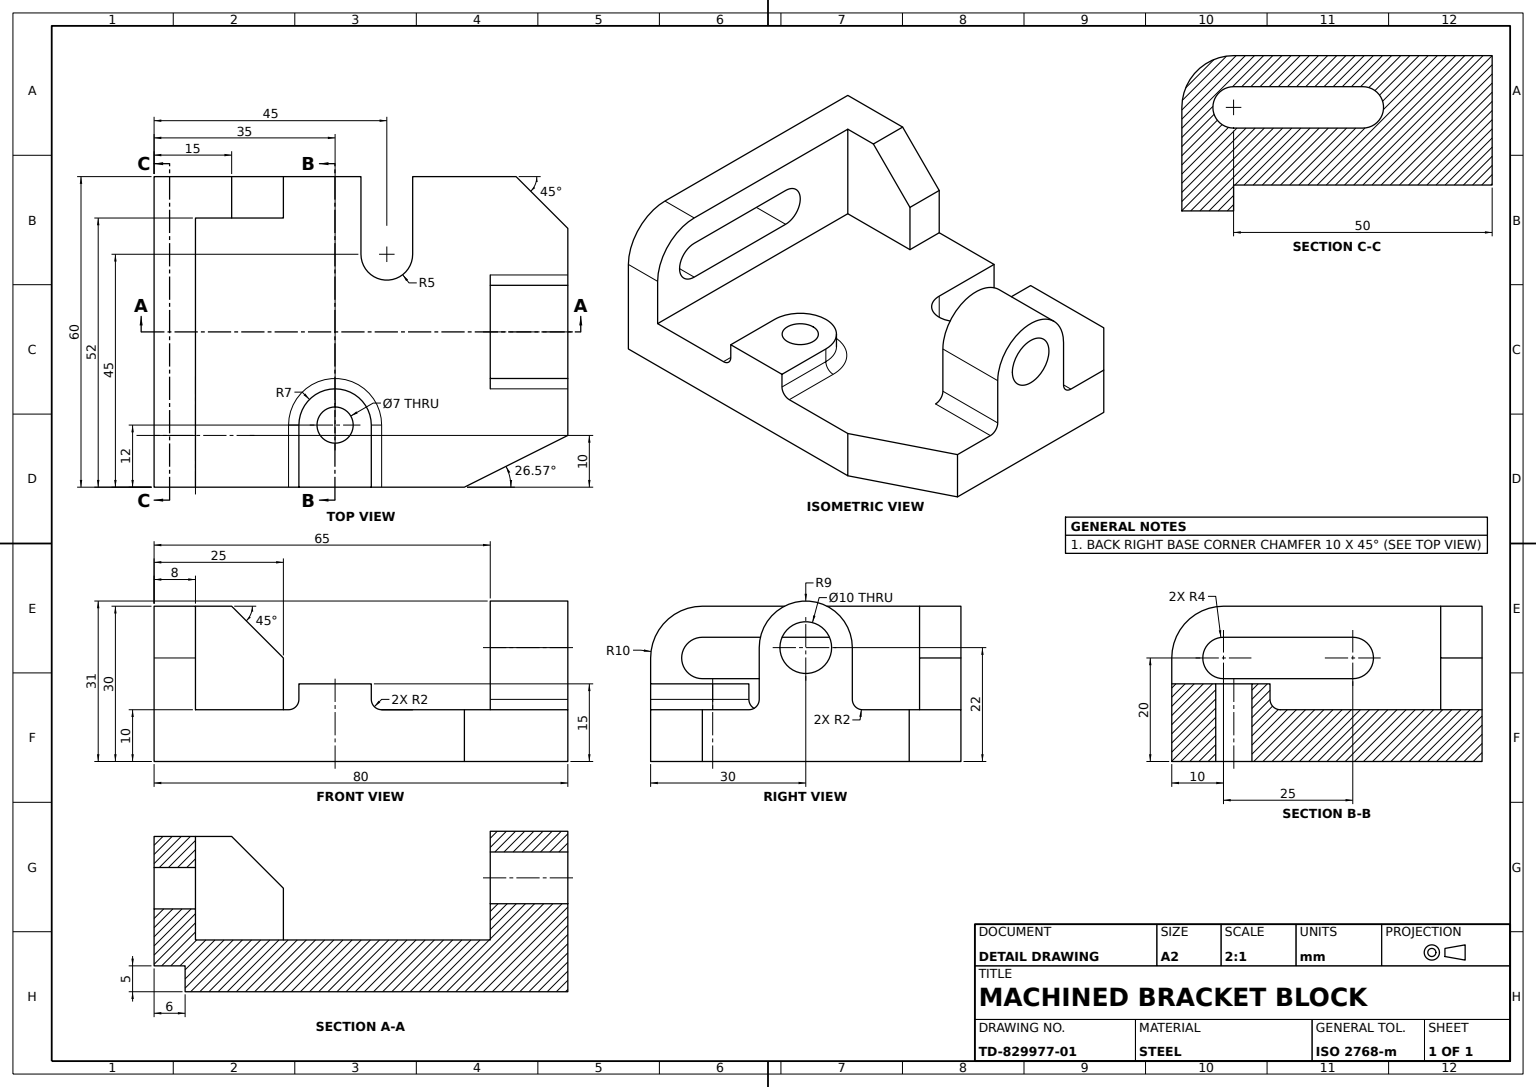
SolidWorks part; units mm, degrees
material "Plain Carbon Steel"
ref_plane "Front Plane" through (0, 0, 0) normal (0, 0, 1) x (1, 0, 0)
ref_plane "Top Plane" through (0, 0, 0) normal (0, 1, 0) x (1, 0, 0)
ref_plane "Right Plane" through (0, 0, 0) normal (1, 0, 0) x (0, 0, -1)
sketch "Base Plate Sketch" plane through (0, 0, 0) normal (0, 1, 0) x (1, 0, 0)
  line L0 (0, 0) -> (0, 30)
  line L1 (0, 30) -> (40, 30)
  line L2 (40, 30) -> (40, 15)
  line L3 (50, 15) -> (50, 30)
  line L4 (50, 30) -> (80, 30)
  line L5 (80, 30) -> (80, -20)
  line L6 (80, -20) -> (60, -30)
  line L7 (60, -30) -> (0, -30)
  line L8 (0, -30) -> (0, 0)
  arc A0 (40, 15) -> (50, 15) centre (45, 15) ccw
  dimension "D3" = 5
  dimension "D1" = 80
  dimension "D2" = 15
  dimension "D4" = 60
  dimension "D5" = 30
  dimension "D6" = 10
  dimension "D7" = 20
  dimension "D8" = 30
extrude "Base Plate 80x60x10" add sketch "Base Plate Sketch" along normal blind 10
chamfer "Base Corner Chamfer 10" distance 10 angle 45 1 edges at (80, 5, -30)
sketch "Slotted Wall Sketch" plane through (0, 0, 0) normal (-1, 0, 0) x (0, 0, 1)
  line L1 (20, 30) -> (-30, 30)
  line L2 (-30, 30) -> (-30, 10)
  line L3 (-30, 10) -> (-30, 0) construction
  line L4 (-30, 10) -> (30, 10)
  line L9 (20, 20) -> (-5, 20) construction
  line L10 (20, 16) -> (-5, 16)
  line L11 (20, 24) -> (-5, 24)
  line L12 (30, 20) -> (30, 10)
  arc A0 (30, 20) -> (20, 30) centre (20, 20) ccw
  arc A1 (20, 16) -> (20, 24) centre (20, 20) ccw
  arc A2 (-5, 24) -> (-5, 16) centre (-5, 20) ccw
  point P18 (7.5, 20)
  dimension "D3" = 10
  dimension "D4" = 4
  dimension "D2" = 20
  dimension "D5" = 10
  dimension "D6" = 25
  dimension "D7" = 12.5
extrude "Slotted Upright Wall" add sketch "Slotted Wall Sketch" against normal blind 8
sketch "Side Block Sketch" plane through (0, 0, -30) normal (0, 0, -1) x (-1, 0, 0)
  line L0 (-8, 30) -> (-25, 30)
  line L1 (-25, 30) -> (-25, 10)
  line L2 (-25, 10) -> (-8, 10)
  line L3 (-8, 10) -> (-8, 30)
  line L4 (0, 20) -> (0, 30) construction
  line L5 (-8, 10) -> (-60, 10) construction
  dimension "D1" = 25
extrude "Side Block 25" add sketch "Side Block Sketch" against normal blind 8
chamfer "Side Block Top Chamfer 10" distance 10 angle 45 1 edges at (25, 30, -26)
sketch "Hole Pad Sketch" plane through (0, 10, 0) normal (0, 1, 0) x (1, 0, 0)
  line L0 (8, -30) -> (60, -30) construction
  line L1 (28, -18) -> (28, -30)
  line L2 (28, -30) -> (42, -30)
  line L3 (42, -30) -> (42, -18)
  arc A0 (42, -18) -> (28, -18) centre (35, -18) ccw
  dimension "D2" = 7
  dimension "D1" = 12
  dimension "D3" = 35
extrude "Hole Pad" add sketch "Hole Pad Sketch" along normal blind 5
sketch "Pad Hole Sketch" plane through (0, 15, 0) normal (0, 1, 0) x (1, 0, 0)
  circle A0 centre (35, -18) radius 3.5
  arc A1 (42, -18) -> (28, -18) centre (35, -18) ccw construction
  dimension "D1" = 7
extrude "Pad Hole Ø7" cut sketch "Pad Hole Sketch" against normal through all
sketch "Pivot Lug Sketch" plane through (80, 0, 0) normal (1, 0, 0) x (0, 0, -1)
  line L0 (-9, 22) -> (-9, 10)
  line L1 (22, 10) -> (-30, 10) construction
  line L2 (-9, 10) -> (9, 10)
  line L3 (9, 10) -> (9, 22)
  line L4 (-20, 10) -> (20, 10) construction
  arc A0 (9, 22) -> (-9, 22) centre (0, 22) ccw
  circle A1 centre (0, 22) radius 5
  dimension "D1" = 9
  dimension "D2" = 10
  dimension "D3" = 12
extrude "Pivot Lug" add sketch "Pivot Lug Sketch" against normal blind 15
fillet "Lug Root Fillet R2" radius 2 5 edges at (28, 10, 24) (35, 10, 11) (42, 10, 24) (72.5, 10, -9) (72.5, 10, 9)
sketch "Relief Groove Sketch" plane through (0, 0, -30) normal (0, 0, -1) x (-1, 0, 0)
  line L1 (0, 0) -> (-6, 0)
  line L2 (0, 0) -> (0, 5)
  line L3 (0, 5) -> (-6, 5)
  line L4 (-6, 0) -> (-6, 5)
  dimension "D1" = 6
  dimension "D2" = 5
extrude "Relief Groove 6x5" cut sketch "Relief Groove Sketch" against normal blind 50
